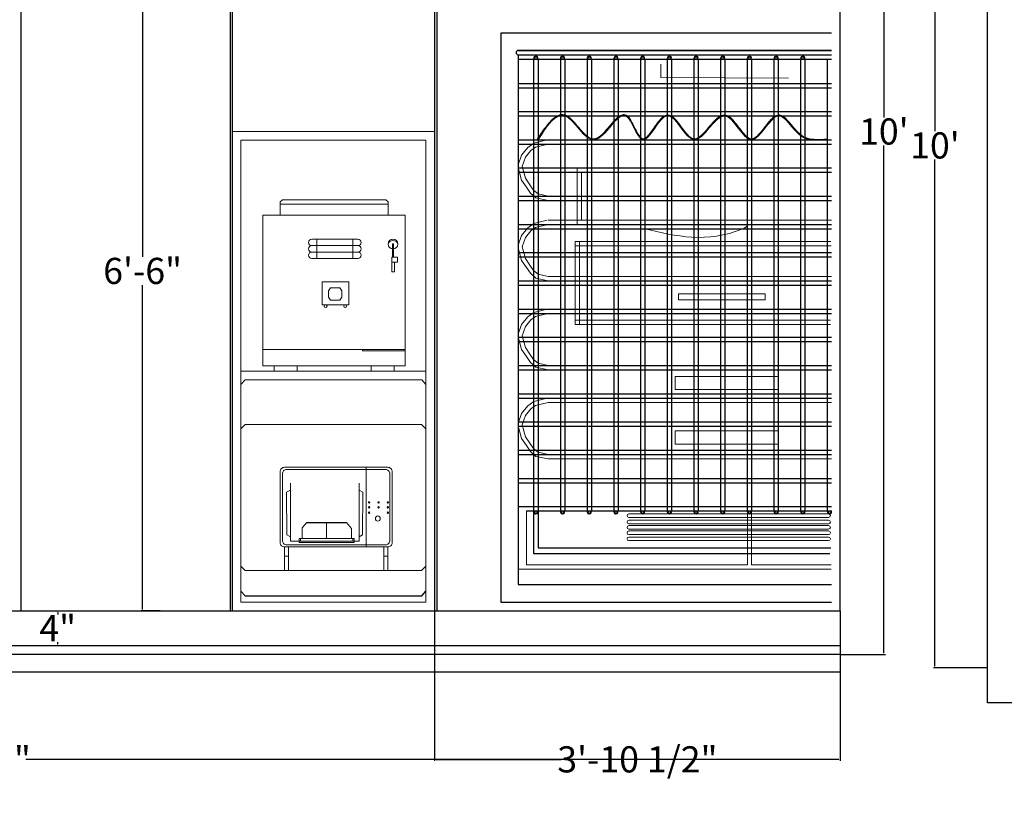
# Model space of a CAD drawing. Units: inches. Extents: x 1686244 to 1686928, y 1936095 to 1936489.
# Tile 5 of 11: x 1686365 to 1686478, y 1936336 to 1936425. Entities that reach past the tile are written whole.
import ezdxf

# ---------------------------------------------------------------- set-up
doc = ezdxf.new("R2010")
doc.units = ezdxf.units.IN
doc.header["$MEASUREMENT"] = 0
for name, color, linetype, lineweight in [('A-ANNO-DIMS', 240, 'Continuous', 18), ('A-ELEV', 7, 'Continuous', 25), ('A-ELEV-PATT', 72, 'Continuous', 13), ('A-FURN', 40, 'Continuous', 18)]:
    doc.layers.add(name, color=color, linetype=linetype, lineweight=lineweight)
doc.styles.get("Standard").update_dxf_attribs({"font": 'arial.ttf'})
doc.dimstyles.get("Standard").update_dxf_attribs({"dimtxt": 3, "dimasz": 0.18, "dimexe": 0.18, "dimexo": 0.0625, "dimgap": 0.09, "dimtad": 0, "dimtih": 1, "dimtoh": 1, "dimzin": 0, "dimdsep": 46, "dimlunit": 4, "dimtxsty": 'Standard', "dimcen": 0.09, "dimadec": 0, "dimazin": 0, "dimtfac": 1, "dimtofl": 0, "dimtmove": 0, "dimatfit": 3, "dimfxl": 1, "dimtolj": 1, "dimtzin": 0, "dimarcsym": 0})

# ---------------------------------------------------------------- blocks, each defined once
blk = doc.blocks.new('*D8')
at = {"layer": 'A-ANNO-DIMS', "color": 0, "lineweight": -2, "transparency": 16777216}
for p, q in [((1686381.35, 1936435.41), (1686379.15, 1936435.41)), ((1686379.33, 1936435.23), (1686379.33, 1936398.03)), ((1686379.33, 1936357.59), (1686379.33, 1936394.79)), ((1686381.35, 1936357.41), (1686379.15, 1936357.41))]:
    blk.add_line(p, q, dxfattribs=at)
at = {"layer": 'A-ANNO-DIMS', "color": 0, "transparency": 16777216}
for points in [[(1686379.3, 1936435.23), (1686379.36, 1936435.23), (1686379.33, 1936435.41)], [(1686379.3, 1936357.59), (1686379.36, 1936357.59), (1686379.33, 1936357.41)]]:
    blk.add_solid(points, dxfattribs=at)
at = {"layer": 'Defpoints', "color": 0, "transparency": 16777216}
for p in [(1686379.33, 1936435.41), (1686381.41, 1936435.41), (1686381.41, 1936357.41)]:
    blk.add_point(p, dxfattribs=at)
at = {"layer": 'A-ANNO-DIMS', "color": 0, "transparency": 16777216, "insert": (1686379.33, 1936396.41), "char_height": 3, "attachment_point": 5}
blk.add_mtext('\\A1;6\'-6"', dxfattribs=at)
blk = doc.blocks.new('*D20')
at = {"layer": 'A-ANNO-DIMS', "color": 0, "lineweight": -2, "transparency": 16777216}
for p, q in [((1686476.2, 1936470.86), (1686470.03, 1936470.86)), ((1686470.21, 1936470.68), (1686470.21, 1936412.44)), ((1686470.21, 1936351.04), (1686470.21, 1936409.19)), ((1686476.2, 1936350.86), (1686470.03, 1936350.86))]:
    blk.add_line(p, q, dxfattribs=at)
at = {"layer": 'A-ANNO-DIMS', "color": 0, "transparency": 16777216}
for points in [[(1686470.18, 1936470.68), (1686470.24, 1936470.68), (1686470.21, 1936470.86)], [(1686470.18, 1936351.04), (1686470.24, 1936351.04), (1686470.21, 1936350.86)]]:
    blk.add_solid(points, dxfattribs=at)
at = {"layer": 'Defpoints', "color": 0, "transparency": 16777216}
for p in [(1686476.26, 1936470.86), (1686470.21, 1936350.86), (1686476.26, 1936350.86)]:
    blk.add_point(p, dxfattribs=at)
at = {"layer": 'A-ANNO-DIMS', "color": 0, "transparency": 16777216, "insert": (1686470.21, 1936410.81), "char_height": 3, "attachment_point": 5}
blk.add_mtext("\\A1;10'", dxfattribs=at)
blk = doc.blocks.new('*D57')
at = {"layer": 'A-ANNO-DIMS', "color": 0, "lineweight": -2, "transparency": 16777216}
for p, q in [((1686368.79, 1936357.41), (1686369.77, 1936357.41)), ((1686369.59, 1936357.23), (1686369.59, 1936357)), ((1686368.79, 1936353.41), (1686369.77, 1936353.41)), ((1686369.59, 1936353.59), (1686369.59, 1936353.82))]:
    blk.add_line(p, q, dxfattribs=at)
at = {"layer": 'A-ANNO-DIMS', "color": 0, "transparency": 16777216}
for points in [[(1686369.56, 1936357.23), (1686369.62, 1936357.23), (1686369.59, 1936357.41)], [(1686369.56, 1936353.59), (1686369.62, 1936353.59), (1686369.59, 1936353.41)]]:
    blk.add_solid(points, dxfattribs=at)
at = {"layer": 'Defpoints', "color": 0, "transparency": 16777216}
for p in [(1686368.73, 1936357.41), (1686369.59, 1936357.41), (1686368.73, 1936353.41)]:
    blk.add_point(p, dxfattribs=at)
at = {"layer": 'A-ANNO-DIMS', "color": 0, "transparency": 16777216, "insert": (1686369.59, 1936355.41), "char_height": 3, "attachment_point": 5}
blk.add_mtext('\\A1;4"', dxfattribs=at)
blk = doc.blocks.new('*D64')
at = {"layer": 'A-ANNO-DIMS', "color": 0, "lineweight": -2, "transparency": 16777216}
for p, q in [((1686459.35, 1936472.41), (1686464.53, 1936472.41)), ((1686464.35, 1936472.23), (1686464.35, 1936414.03)), ((1686464.35, 1936352.59), (1686464.35, 1936410.79)), ((1686459.35, 1936352.41), (1686464.53, 1936352.41))]:
    blk.add_line(p, q, dxfattribs=at)
at = {"layer": 'A-ANNO-DIMS', "color": 0, "transparency": 16777216}
for points in [[(1686464.32, 1936472.23), (1686464.38, 1936472.23), (1686464.35, 1936472.41)], [(1686464.32, 1936352.59), (1686464.38, 1936352.59), (1686464.35, 1936352.41)]]:
    blk.add_solid(points, dxfattribs=at)
at = {"layer": 'Defpoints', "color": 0, "transparency": 16777216}
for p in [(1686459.29, 1936472.41), (1686459.29, 1936352.41), (1686464.35, 1936352.41)]:
    blk.add_point(p, dxfattribs=at)
at = {"layer": 'A-ANNO-DIMS', "color": 0, "transparency": 16777216, "insert": (1686464.35, 1936412.41), "char_height": 3, "attachment_point": 5}
blk.add_mtext("\\A1;10'", dxfattribs=at)
blk = doc.blocks.new('*D87')
at = {"layer": 'A-ANNO-DIMS', "color": 0, "lineweight": -2, "transparency": 16777216}
for p, q in [((1686262.35, 1936350.35), (1686262.35, 1936340.18)), ((1686459.35, 1936350.35), (1686459.35, 1936340.18)), ((1686262.53, 1936340.36), (1686355.75, 1936340.36)), ((1686459.17, 1936340.36), (1686365.95, 1936340.36))]:
    blk.add_line(p, q, dxfattribs=at)
at = {"layer": 'A-ANNO-DIMS', "color": 0, "transparency": 16777216}
for points in [[(1686262.53, 1936340.39), (1686262.53, 1936340.33), (1686262.35, 1936340.36)], [(1686459.17, 1936340.39), (1686459.17, 1936340.33), (1686459.35, 1936340.36)]]:
    blk.add_solid(points, dxfattribs=at)
at = {"layer": 'Defpoints', "color": 0, "transparency": 16777216}
for p in [(1686262.35, 1936350.41), (1686459.35, 1936350.41), (1686459.35, 1936340.36)]:
    blk.add_point(p, dxfattribs=at)
at = {"layer": 'A-ANNO-DIMS', "color": 0, "transparency": 16777216, "insert": (1686360.85, 1936340.36), "char_height": 3, "attachment_point": 5}
blk.add_mtext('\\A1;16\'-5"', dxfattribs=at)
blk = doc.blocks.new('*D91')
at = {"layer": 'A-ANNO-DIMS', "color": 0, "lineweight": -2, "transparency": 16777216}
for p, q in [((1686412.81, 1936357.35), (1686412.81, 1936340.18)), ((1686459.35, 1936357.35), (1686459.35, 1936340.18)), ((1686412.99, 1936340.36), (1686427.34, 1936340.36)), ((1686459.17, 1936340.36), (1686444.82, 1936340.36))]:
    blk.add_line(p, q, dxfattribs=at)
at = {"layer": 'A-ANNO-DIMS', "color": 0, "transparency": 16777216}
for points in [[(1686412.99, 1936340.39), (1686412.99, 1936340.33), (1686412.81, 1936340.36)], [(1686459.17, 1936340.39), (1686459.17, 1936340.33), (1686459.35, 1936340.36)]]:
    blk.add_solid(points, dxfattribs=at)
at = {"layer": 'Defpoints', "color": 0, "transparency": 16777216}
for p in [(1686412.81, 1936357.41), (1686459.35, 1936357.41), (1686459.35, 1936340.36)]:
    blk.add_point(p, dxfattribs=at)
at = {"layer": 'A-ANNO-DIMS', "color": 0, "transparency": 16777216, "insert": (1686436.08, 1936340.36), "char_height": 3, "attachment_point": 5}
blk.add_mtext('\\A1;3\'-10 1/2"', dxfattribs=at)

msp = doc.modelspace()

# ---------------------------------------------------------------- linework, layer by layer
at = {"layer": 'A-ELEV'}
for p, q in [((1686365.353, 1936467.412), (1686365.353, 1936357.412)), ((1686389.353, 1936467.412), (1686389.353, 1936357.412)), ((1686389.609, 1936467.412), (1686389.609, 1936357.412)), ((1686412.809, 1936467.412), (1686412.809, 1936357.412)), ((1686413.059, 1936467.412), (1686413.059, 1936357.412)), ((1686422.413, 1936421.704), (1686458.353, 1936421.704)), ((1686422.413, 1936421.204), (1686458.353, 1936421.204)), ((1686422.413, 1936420.704), (1686458.353, 1936420.704)), ((1686424.183, 1936420.704), (1686424.183, 1936368.86)), ((1686424.683, 1936420.704), (1686424.683, 1936368.86)), ((1686427.244, 1936420.704), (1686427.244, 1936368.86)), ((1686427.744, 1936420.704), (1686427.744, 1936368.86)), ((1686430.305, 1936420.704), (1686430.305, 1936368.86)), ((1686430.805, 1936420.704), (1686430.805, 1936368.86)), ((1686433.366, 1936420.704), (1686433.366, 1936368.86)), ((1686433.866, 1936420.704), (1686433.866, 1936368.86)), ((1686436.427, 1936420.704), (1686436.427, 1936368.86)), ((1686436.927, 1936420.704), (1686436.927, 1936368.86)), ((1686439.488, 1936420.704), (1686439.488, 1936368.86)), ((1686439.988, 1936420.704), (1686439.988, 1936368.86)), ((1686442.549, 1936420.704), (1686442.549, 1936368.86)), ((1686443.049, 1936420.704), (1686443.049, 1936368.86)), ((1686445.609, 1936420.704), (1686445.609, 1936368.86)), ((1686446.109, 1936420.704), (1686446.109, 1936368.86)), ((1686448.67, 1936420.704), (1686448.67, 1936368.86)), ((1686449.17, 1936420.704), (1686449.17, 1936368.86)), ((1686451.731, 1936420.704), (1686451.731, 1936368.86)), ((1686452.231, 1936420.704), (1686452.231, 1936368.86)), ((1686454.792, 1936420.704), (1686454.792, 1936368.86)), ((1686455.292, 1936420.704), (1686455.292, 1936368.86)), ((1686457.853, 1936420.704), (1686457.853, 1936368.86)), ((1686422.413, 1936417.909), (1686458.353, 1936417.909)), ((1686422.413, 1936417.409), (1686458.353, 1936417.409)), ((1686422.413, 1936414.704), (1686458.353, 1936414.704)), ((1686422.413, 1936414.204), (1686458.353, 1936414.204)), ((1686422.413, 1936411.465), (1686458.353, 1936411.465)), ((1686422.413, 1936410.965), (1686458.353, 1936410.965)), ((1686422.413, 1936408.226), (1686458.353, 1936408.226)), ((1686422.413, 1936407.726), (1686458.353, 1936407.726)), ((1686422.413, 1936404.987), (1686458.353, 1936404.987)), ((1686422.413, 1936404.487), (1686458.353, 1936404.487)), ((1686422.413, 1936401.748), (1686458.353, 1936401.748)), ((1686422.413, 1936401.248), (1686458.353, 1936401.248)), ((1686422.413, 1936398.51), (1686458.353, 1936398.51)), ((1686422.413, 1936398.01), (1686458.353, 1936398.01)), ((1686422.413, 1936395.271), (1686458.353, 1936395.271)), ((1686422.413, 1936394.771), (1686458.353, 1936394.771)), ((1686422.413, 1936392.032), (1686458.353, 1936392.032)), ((1686422.413, 1936391.532), (1686458.353, 1936391.532)), ((1686422.413, 1936388.793), (1686458.353, 1936388.793)), ((1686422.413, 1936388.293), (1686458.353, 1936388.293)), ((1686422.413, 1936385.554), (1686458.353, 1936385.554)), ((1686422.413, 1936385.054), (1686458.353, 1936385.054)), ((1686391.075, 1936383.912), (1686390.609, 1936383.372)), ((1686422.413, 1936382.315), (1686458.353, 1936382.315)), ((1686422.413, 1936381.815), (1686458.353, 1936381.815)), ((1686422.413, 1936379.076), (1686458.353, 1936379.076)), ((1686422.413, 1936378.576), (1686458.353, 1936378.576)), ((1686422.413, 1936375.838), (1686458.353, 1936375.838)), ((1686422.413, 1936375.338), (1686458.353, 1936375.338)), ((1686422.413, 1936372.599), (1686458.353, 1936372.599)), ((1686422.413, 1936372.099), (1686458.353, 1936372.099)), ((1686422.413, 1936369.36), (1686458.353, 1936369.36)), ((1686423.367, 1936368.86), (1686458.353, 1936368.86)), ((1686424.183, 1936368.86), (1686424.183, 1936364.397)), ((1686424.683, 1936369.36), (1686424.683, 1936364.626)), ((1686424.183, 1936364.397), (1686424.183, 1936363.992)), ((1686424.683, 1936364.626), (1686458.265, 1936364.626)), ((1686424.183, 1936363.992), (1686458.172, 1936363.992)), ((1686422.413, 1936360.412), (1686458.353, 1936360.412)), ((1686391.075, 1936359.109), (1686390.609, 1936359.648)), ((1686391.075, 1936359.109), (1686411.343, 1936359.109)), ((1686411.343, 1936359.109), (1686411.809, 1936359.648)), ((1686420.413, 1936358.412), (1686458.353, 1936358.412)), ((1686459.353, 1936357.412), (1686459.353, 1936350.412)), ((1686262.353, 1936353.412), (1686459.353, 1936353.412)), ((1686262.353, 1936352.412), (1686459.353, 1936352.412)), ((1686262.353, 1936350.412), (1686459.353, 1936350.412))]:
    msp.add_line(p, q, dxfattribs=at)
for points in [[(1686691.259, 1936346.864), (1686476.258, 1936346.864), (1686476.258, 1936474.864), (1686691.259, 1936474.864)], [(1686459.353, 1936357.412), (1686459.353, 1936467.412), (1686262.353, 1936467.412), (1686262.353, 1936357.412)]]:
    msp.add_lwpolyline(points, close=True, dxfattribs=at)
for points in [[(1686458.353, 1936423.704), (1686420.413, 1936423.704), (1686420.413, 1936358.412)], [(1686458.353, 1936421.704), (1686422.413, 1936421.704)], [(1686422.413, 1936421.204), (1686422.413, 1936360.412)]]:
    msp.add_lwpolyline(points, dxfattribs=at)
for centre in [(1686424.438, 1936420.891), (1686427.5, 1936420.891), (1686430.563, 1936420.891), (1686433.626, 1936420.891), (1686436.688, 1936420.891), (1686439.751, 1936420.891), (1686442.814, 1936420.891), (1686445.877, 1936420.891), (1686448.939, 1936420.891), (1686452.002, 1936420.891), (1686455.065, 1936420.891), (1686424.438, 1936368.673), (1686427.5, 1936368.673), (1686430.563, 1936368.673), (1686433.626, 1936368.673), (1686436.688, 1936368.673), (1686439.751, 1936368.673), (1686442.814, 1936368.673), (1686445.877, 1936368.673), (1686448.939, 1936368.673), (1686452.002, 1936368.673), (1686455.065, 1936368.673), (1686458.128, 1936368.673)]:
    msp.add_circle(centre, 0.187, dxfattribs=at)
for centre, start, end in [((1686422.413, 1936421.454), 90, 270), ((1686424.433, 1936420.704), 0, 180), ((1686427.494, 1936420.704), 0, 180), ((1686430.555, 1936420.704), 0, 180), ((1686433.616, 1936420.704), 0, 180), ((1686436.677, 1936420.704), 0, 180), ((1686439.738, 1936420.704), 0, 180), ((1686442.799, 1936420.704), 0, 180), ((1686445.859, 1936420.704), 0, 180), ((1686448.92, 1936420.704), 0, 180), ((1686451.981, 1936420.704), 0, 180), ((1686455.042, 1936420.704), 0, 180), ((1686424.433, 1936368.86), 180, 0), ((1686427.494, 1936368.86), 180, 0), ((1686430.555, 1936368.86), 180, 0), ((1686433.616, 1936368.86), 180, 0), ((1686436.677, 1936368.86), 180, 0), ((1686439.738, 1936368.86), 180, 0), ((1686442.799, 1936368.86), 180, 0), ((1686445.859, 1936368.86), 180, 0), ((1686448.92, 1936368.86), 180, 0), ((1686451.981, 1936368.86), 180, 0), ((1686455.042, 1936368.86), 180, 0), ((1686458.103, 1936368.86), 180, 0)]:
    msp.add_arc(centre, 0.25, start, end, dxfattribs=at)
at = {"layer": 'A-ELEV-PATT'}
for p, q in [((1686438.763, 1936420.144), (1686438.763, 1936418.618)), ((1686453.413, 1936418.543), (1686438.763, 1936418.618)), ((1686458.353, 1936411.465), (1686425.837, 1936411.465)), ((1686458.353, 1936410.965), (1686425.837, 1936410.965)), ((1686436.949, 1936411.62), (1686436.949, 1936399.785)), ((1686448.67, 1936410.965), (1686448.67, 1936402.248)), ((1686457.853, 1936408.226), (1686429.184, 1936408.226)), ((1686429.184, 1936408.226), (1686429.184, 1936401.748)), ((1686457.853, 1936407.726), (1686429.684, 1936407.726)), ((1686429.684, 1936407.726), (1686429.684, 1936402.248)), ((1686458.353, 1936404.987), (1686425.837, 1936404.987)), ((1686458.353, 1936404.487), (1686425.837, 1936404.487)), ((1686458.353, 1936402.248), (1686425.837, 1936402.248)), ((1686458.353, 1936401.748), (1686425.837, 1936401.748)), ((1686429.184, 1936401.748), (1686458.353, 1936401.748)), ((1686429.684, 1936402.248), (1686458.353, 1936402.248)), ((1686458.282, 1936399.785), (1686428.93, 1936399.785)), ((1686428.93, 1936399.785), (1686428.93, 1936390.251)), ((1686458.291, 1936399.285), (1686428.93, 1936399.285)), ((1686429.43, 1936399.785), (1686429.43, 1936390.251)), ((1686458.353, 1936395.771), (1686425.837, 1936395.771)), ((1686458.353, 1936395.271), (1686425.837, 1936395.271)), ((1686458.353, 1936392.032), (1686425.837, 1936392.032)), ((1686458.353, 1936391.532), (1686425.837, 1936391.532)), ((1686428.93, 1936390.751), (1686458.227, 1936390.751)), ((1686428.93, 1936390.251), (1686458.227, 1936390.251)), ((1686458.353, 1936385.554), (1686425.337, 1936385.554)), ((1686458.353, 1936385.054), (1686425.837, 1936385.054)), ((1686458.353, 1936381.815), (1686425.837, 1936381.815)), ((1686458.353, 1936381.315), (1686425.837, 1936381.315)), ((1686458.353, 1936375.338), (1686425.837, 1936375.338)), ((1686458.353, 1936374.838), (1686425.837, 1936374.838)), ((1686423.367, 1936362.687), (1686423.367, 1936368.86)), ((1686449.17, 1936368.86), (1686449.17, 1936362.687)), ((1686435.105, 1936368.531), (1686458.007, 1936368.531)), ((1686435.105, 1936368.118), (1686458.007, 1936368.118)), ((1686435.105, 1936367.797), (1686458.007, 1936367.797)), ((1686448.699, 1936362.687), (1686448.699, 1936368.531)), ((1686435.105, 1936367.385), (1686458.007, 1936367.385)), ((1686435.105, 1936367.19), (1686458.007, 1936367.19)), ((1686435.105, 1936366.777), (1686458.007, 1936366.777)), ((1686435.105, 1936366.567), (1686458.007, 1936366.567)), ((1686435.105, 1936366.155), (1686458.007, 1936366.155)), ((1686435.105, 1936365.868), (1686458.007, 1936365.868)), ((1686435.105, 1936365.455), (1686458.007, 1936365.455)), ((1686422.413, 1936362.187), (1686458.325, 1936362.187)), ((1686423.367, 1936362.687), (1686448.699, 1936362.687)), ((1686449.17, 1936362.687), (1686458.325, 1936362.687))]:
    msp.add_line(p, q, dxfattribs=at)
for points in [[(1686425.714, 1936411.45), (1686424.198, 1936411.064), (1686423.514, 1936410.585), (1686422.794, 1936409.697), (1686422.407, 1936408.569)], [(1686425.837, 1936410.965), (1686424.41, 1936410.602), (1686423.858, 1936410.216), (1686423.238, 1936409.451), (1686422.88, 1936408.407)], [(1686425.837, 1936404.487), (1686424.45, 1936404.782), (1686423.807, 1936405.349), (1686423.345, 1936406.016), (1686422.787, 1936406.821), (1686422.397, 1936408.277)], [(1686425.837, 1936404.987), (1686424.683, 1936405.242), (1686424.183, 1936405.683), (1686423.756, 1936406.301), (1686423.248, 1936407.035), (1686422.88, 1936408.407)], [(1686425.714, 1936402.233), (1686424.198, 1936401.848), (1686423.514, 1936401.369), (1686422.794, 1936400.481), (1686422.407, 1936399.352)], [(1686425.837, 1936401.748), (1686424.41, 1936401.386), (1686423.858, 1936400.999), (1686423.238, 1936400.235), (1686422.88, 1936399.19)], [(1686425.837, 1936395.271), (1686424.45, 1936395.565), (1686423.807, 1936396.132), (1686423.345, 1936396.8), (1686422.787, 1936397.605), (1686422.397, 1936399.061)], [(1686425.837, 1936395.771), (1686424.683, 1936396.026), (1686424.183, 1936396.467), (1686423.756, 1936397.084), (1686423.248, 1936397.818), (1686422.88, 1936399.19)], [(1686425.714, 1936392.016), (1686424.198, 1936391.631), (1686423.514, 1936391.152), (1686422.794, 1936390.264), (1686422.407, 1936389.136)], [(1686425.837, 1936391.532), (1686424.41, 1936391.169), (1686423.858, 1936390.783), (1686423.238, 1936390.018), (1686422.88, 1936388.974)], [(1686425.837, 1936385.054), (1686424.45, 1936385.349), (1686423.807, 1936385.916), (1686423.345, 1936386.583), (1686422.787, 1936387.388), (1686422.397, 1936388.844)], [(1686425.837, 1936385.554), (1686424.683, 1936385.809), (1686424.183, 1936386.25), (1686423.756, 1936386.868), (1686423.248, 1936387.602), (1686422.88, 1936388.974)], [(1686425.714, 1936381.8), (1686424.198, 1936381.415), (1686423.514, 1936380.936), (1686422.794, 1936380.048), (1686422.407, 1936378.919)], [(1686425.837, 1936381.315), (1686424.41, 1936380.953), (1686423.858, 1936380.566), (1686423.238, 1936379.802), (1686422.88, 1936378.757)], [(1686425.837, 1936374.838), (1686424.45, 1936375.132), (1686423.807, 1936375.699), (1686423.345, 1936376.366), (1686422.787, 1936377.172), (1686422.397, 1936378.628)], [(1686425.837, 1936375.338), (1686424.683, 1936375.593), (1686424.183, 1936376.034), (1686423.756, 1936376.651), (1686423.248, 1936377.385), (1686422.88, 1936378.757)]]:
    msp.add_lwpolyline(points, dxfattribs=at)
for points in [[(1686440.784, 1936393.79), (1686450.756, 1936393.79), (1686450.756, 1936393.104), (1686440.784, 1936393.104)], [(1686440.405, 1936384.298), (1686452.231, 1936384.298), (1686452.231, 1936382.8), (1686440.405, 1936382.8)], [(1686440.405, 1936378.041), (1686452.231, 1936378.041), (1686452.231, 1936376.543), (1686440.405, 1936376.543)]]:
    msp.add_lwpolyline(points, close=True, dxfattribs=at)
for centre, start, end in [((1686435.105, 1936368.324), 90, 270), ((1686435.105, 1936367.591), 90, 270), ((1686458.007, 1936368.324), 270, 90), ((1686458.007, 1936367.591), 270, 90), ((1686435.105, 1936366.983), 90, 270), ((1686435.105, 1936366.361), 90, 270), ((1686458.007, 1936366.983), 270, 90), ((1686458.007, 1936366.361), 270, 90), ((1686435.105, 1936365.662), 90, 270), ((1686458.007, 1936365.662), 270, 90)]:
    msp.add_arc(centre, 0.206, start, end, dxfattribs=at)
for points, knots in [([(1686424.6, 1936411.52), (1686424.753, 1936411.753), (1686424.906, 1936411.986), (1686425.367, 1936412.667), (1686425.675, 1936413.097), (1686426.257, 1936413.758), (1686426.53, 1936414.009), (1686427.035, 1936414.295), (1686427.267, 1936414.364), (1686427.736, 1936414.339), (1686427.969, 1936414.235), (1686428.417, 1936413.909), (1686428.635, 1936413.69), (1686429.072, 1936413.206), (1686429.291, 1936412.941), (1686429.782, 1936412.375), (1686430.055, 1936412.08), (1686430.533, 1936411.711), (1686430.738, 1936411.602), (1686431.091, 1936411.541), (1686431.244, 1936411.559), (1686431.686, 1936411.748), (1686431.988, 1936412.013), (1686432.59, 1936412.656), (1686432.892, 1936413.033), (1686433.381, 1936413.597), (1686433.573, 1936413.805), (1686433.925, 1936414.116), (1686434.086, 1936414.229), (1686434.396, 1936414.349), (1686434.547, 1936414.365), (1686434.834, 1936414.276), (1686434.964, 1936414.176), (1686435.201, 1936413.909), (1686435.31, 1936413.742), (1686435.624, 1936413.2), (1686435.817, 1936412.777), (1686436.142, 1936412.162), (1686436.273, 1936411.94), (1686436.484, 1936411.689), (1686436.564, 1936411.621), (1686436.71, 1936411.552), (1686436.773, 1936411.55), (1686436.931, 1936411.601), (1686437.022, 1936411.659), (1686437.216, 1936411.83), (1686437.318, 1936411.943), (1686437.679, 1936412.388), (1686437.949, 1936412.804), (1686438.409, 1936413.444), (1686438.593, 1936413.684), (1686438.926, 1936414.026), (1686439.074, 1936414.148), (1686439.344, 1936414.281), (1686439.464, 1936414.312), (1686439.702, 1936414.305), (1686439.82, 1936414.27), (1686440.143, 1936414.105), (1686440.342, 1936413.92), (1686440.733, 1936413.476), (1686440.925, 1936413.216), (1686441.364, 1936412.619), (1686441.611, 1936412.28), (1686442.049, 1936411.819), (1686442.24, 1936411.667), (1686442.578, 1936411.541), (1686442.73, 1936411.548), (1686443.068, 1936411.683), (1686443.248, 1936411.812), (1686443.778, 1936412.296), (1686444.138, 1936412.748), (1686444.781, 1936413.499), (1686445.064, 1936413.811), (1686445.524, 1936414.153), (1686445.698, 1936414.246), (1686446.011, 1936414.314), (1686446.148, 1936414.311), (1686446.41, 1936414.237), (1686446.535, 1936414.169), (1686447.02, 1936413.815), (1686447.357, 1936413.368), (1686448.026, 1936412.477), (1686448.358, 1936412.033), (1686448.808, 1936411.676), (1686448.938, 1936411.605), (1686449.184, 1936411.551), (1686449.304, 1936411.568), (1686449.562, 1936411.684), (1686449.7, 1936411.784), (1686449.981, 1936412.044), (1686450.124, 1936412.204), (1686450.594, 1936412.775), (1686450.924, 1936413.246), (1686451.439, 1936413.833), (1686451.621, 1936414.014), (1686451.954, 1936414.233), (1686452.104, 1936414.294), (1686452.409, 1936414.317), (1686452.559, 1936414.275), (1686452.843, 1936414.124), (1686452.979, 1936414.016), (1686453.374, 1936413.64), (1686453.629, 1936413.316), (1686454.164, 1936412.669), (1686454.441, 1936412.347), (1686454.975, 1936411.91), (1686455.229, 1936411.77), (1686455.763, 1936411.583), (1686456.043, 1936411.533), (1686456.817, 1936411.477), (1686457.328, 1936411.52), (1686457.844, 1936411.565)], [0, 0, 0, 0, 0.6198497, 0.6198497, 1.8595491, 1.8595491, 2.9317453, 2.9317453, 3.7773121, 3.7773121, 4.6228788, 4.6228788, 5.4684455, 5.4684455, 6.3140123, 6.3140123, 7.3654424, 7.3654424, 8.1736983, 8.1736983, 8.812576, 8.812576, 9.9067512, 9.9067512, 11.0009263, 11.0009263, 11.7236696, 11.7236696, 12.3447229, 12.3447229, 12.8877348, 12.8877348, 13.4307466, 13.4307466, 13.9737585, 13.9737585, 15.0258606, 15.0258606, 15.7385229, 15.7385229, 16.195193, 16.195193, 16.6560278, 16.6560278, 17.1168626, 17.1168626, 17.5776974, 17.5776974, 18.6933699, 18.6933699, 19.4222939, 19.4222939, 19.9794482, 19.9794482, 20.3901997, 20.3901997, 20.8009512, 20.8009512, 21.5807194, 21.5807194, 22.3604876, 22.3604876, 23.3657967, 23.3657967, 24.1584136, 24.1584136, 24.8711455, 24.8711455, 25.5838774, 25.5838774, 26.9255116, 26.9255116, 27.9769724, 27.9769724, 28.5946697, 28.5946697, 29.0495877, 29.0495877, 29.5045058, 29.5045058, 30.8620561, 30.8620561, 32.2196063, 32.2196063, 32.798175, 32.798175, 33.3767438, 33.3767438, 33.9553125, 33.9553125, 34.5338812, 34.5338812, 35.8487479, 35.8487479, 36.5727796, 36.5727796, 37.1250725, 37.1250725, 37.6773653, 37.6773653, 38.2296582, 38.2296582, 39.294376, 39.294376, 40.3590938, 40.3590938, 41.2411052, 41.2411052, 42.1231167, 42.1231167, 43.5982821, 43.5982821, 43.5982821, 43.5982821]), ([(1686424.621, 1936411.506), (1686424.774, 1936411.739), (1686424.927, 1936411.972), (1686425.387, 1936412.652), (1686425.695, 1936413.081), (1686426.29, 1936413.758), (1686426.578, 1936414.018), (1686427.097, 1936414.291), (1686427.328, 1936414.348), (1686427.792, 1936414.295), (1686428.021, 1936414.177), (1686428.468, 1936413.828), (1686428.688, 1936413.598), (1686429.321, 1936412.884), (1686429.736, 1936412.351), (1686430.369, 1936411.791), (1686430.588, 1936411.645), (1686430.977, 1936411.519), (1686431.148, 1936411.515), (1686431.612, 1936411.664), (1686431.919, 1936411.915), (1686432.531, 1936412.547), (1686432.838, 1936412.928), (1686433.342, 1936413.515), (1686433.542, 1936413.738), (1686433.911, 1936414.074), (1686434.081, 1936414.198), (1686434.379, 1936414.317), (1686434.508, 1936414.336), (1686434.76, 1936414.283), (1686434.878, 1936414.21), (1686435.095, 1936414.002), (1686435.196, 1936413.866), (1686435.53, 1936413.342), (1686435.746, 1936412.863), (1686436.093, 1936412.198), (1686436.224, 1936411.971), (1686436.443, 1936411.693), (1686436.533, 1936411.611), (1686436.699, 1936411.527), (1686436.776, 1936411.523), (1686436.954, 1936411.584), (1686437.054, 1936411.651), (1686437.266, 1936411.846), (1686437.377, 1936411.972), (1686437.767, 1936412.469), (1686438.059, 1936412.926), (1686438.53, 1936413.559), (1686438.703, 1936413.772), (1686439.057, 1936414.106), (1686439.239, 1936414.228), (1686439.58, 1936414.302), (1686439.733, 1936414.277), (1686440.021, 1936414.146), (1686440.16, 1936414.042), (1686440.557, 1936413.667), (1686440.81, 1936413.329), (1686441.318, 1936412.64), (1686441.571, 1936412.289), (1686442.008, 1936411.823), (1686442.191, 1936411.671), (1686442.542, 1936411.518), (1686442.71, 1936411.517), (1686443.073, 1936411.654), (1686443.264, 1936411.791), (1686443.654, 1936412.15), (1686443.853, 1936412.371), (1686444.411, 1936413.022), (1686444.772, 1936413.479), (1686445.34, 1936413.999), (1686445.545, 1936414.147), (1686445.897, 1936414.275), (1686446.04, 1936414.294), (1686446.429, 1936414.229), (1686446.659, 1936414.07), (1686447.106, 1936413.641), (1686447.323, 1936413.368), (1686447.791, 1936412.751), (1686448.042, 1936412.403), (1686448.476, 1936411.912), (1686448.66, 1936411.74), (1686448.977, 1936411.562), (1686449.108, 1936411.528), (1686449.374, 1936411.56), (1686449.512, 1936411.625), (1686449.801, 1936411.834), (1686449.95, 1936411.978), (1686450.568, 1936412.664), (1686451.041, 1936413.402), (1686451.676, 1936414.019), (1686451.836, 1936414.143), (1686452.127, 1936414.269), (1686452.256, 1936414.293), (1686452.508, 1936414.264), (1686452.63, 1936414.216), (1686453.054, 1936413.958), (1686453.343, 1936413.623), (1686453.947, 1936412.894), (1686454.259, 1936412.499), (1686454.782, 1936412.024), (1686454.978, 1936411.886), (1686455.387, 1936411.679), (1686455.599, 1936411.608), (1686456.258, 1936411.463), (1686456.726, 1936411.462), (1686457.417, 1936411.503), (1686457.631, 1936411.521), (1686457.846, 1936411.54)], [0, 0, 0, 0, 0.6195688, 0.6195688, 1.8587065, 1.8587065, 2.9947443, 2.9947443, 3.8509643, 3.8509643, 4.7071842, 4.7071842, 5.5634041, 5.5634041, 7.1611739, 7.1611739, 8.0023315, 8.0023315, 8.6973238, 8.6973238, 9.8074601, 9.8074601, 10.9175963, 10.9175963, 11.6720865, 11.6720865, 12.3339957, 12.3339957, 12.8235788, 12.8235788, 13.3131619, 13.3131619, 13.802745, 13.802745, 14.9803996, 14.9803996, 15.6853017, 15.6853017, 16.1753468, 16.1753468, 16.6653918, 16.6653918, 17.1554369, 17.1554369, 17.645482, 17.645482, 18.8425445, 18.8425445, 19.5256228, 19.5256228, 20.208701, 20.208701, 20.7473398, 20.7473398, 21.2859785, 21.2859785, 22.3167922, 22.3167922, 23.3476058, 23.3476058, 24.0974736, 24.0974736, 24.8473414, 24.8473414, 25.5972092, 25.5972092, 26.347077, 26.347077, 27.6906732, 27.6906732, 28.4455681, 28.4455681, 28.9435164, 28.9435164, 29.8123427, 29.8123427, 30.6811689, 30.6811689, 31.706993, 31.706993, 32.4760399, 32.4760399, 33.0780575, 33.0780575, 33.6800751, 33.6800751, 34.2820927, 34.2820927, 36.1683264, 36.1683264, 36.8029374, 36.8029374, 37.2799861, 37.2799861, 37.7570348, 37.7570348, 38.9828061, 38.9828061, 40.2085774, 40.2085774, 40.9022496, 40.9022496, 41.5959217, 41.5959217, 42.9832661, 42.9832661, 43.5982821, 43.5982821, 43.5982821, 43.5982821]), ([(1686424.642, 1936411.492), (1686424.795, 1936411.725), (1686424.948, 1936411.958), (1686425.407, 1936412.637), (1686425.714, 1936413.065), (1686426.332, 1936413.767), (1686426.642, 1936414.042), (1686427.185, 1936414.292), (1686427.416, 1936414.331), (1686427.878, 1936414.233), (1686428.105, 1936414.093), (1686428.555, 1936413.707), (1686428.779, 1936413.462), (1686429.425, 1936412.716), (1686429.851, 1936412.18), (1686430.493, 1936411.677), (1686430.706, 1936411.56), (1686431.069, 1936411.492), (1686431.22, 1936411.505), (1686431.533, 1936411.622), (1686431.694, 1936411.723), (1686432.331, 1936412.237), (1686432.816, 1936412.874), (1686433.549, 1936413.71), (1686433.811, 1936413.981), (1686434.225, 1936414.242), (1686434.382, 1936414.301), (1686434.653, 1936414.293), (1686434.767, 1936414.249), (1686434.978, 1936414.092), (1686435.077, 1936413.981), (1686435.442, 1936413.474), (1686435.686, 1936412.926), (1686436.086, 1936412.156), (1686436.241, 1936411.888), (1686436.493, 1936411.611), (1686436.587, 1936411.542), (1686436.769, 1936411.496), (1686436.863, 1936411.515), (1686437.07, 1936411.629), (1686437.182, 1936411.726), (1686437.412, 1936411.973), (1686437.53, 1936412.123), (1686437.97, 1936412.721), (1686438.306, 1936413.252), (1686438.821, 1936413.859), (1686438.997, 1936414.031), (1686439.304, 1936414.215), (1686439.434, 1936414.259), (1686439.695, 1936414.259), (1686439.823, 1936414.217), (1686440.246, 1936413.979), (1686440.531, 1936413.647), (1686441.102, 1936412.901), (1686441.386, 1936412.486), (1686441.859, 1936411.933), (1686442.048, 1936411.75), (1686442.372, 1936411.552), (1686442.507, 1936411.507), (1686442.781, 1936411.512), (1686442.921, 1936411.559), (1686443.365, 1936411.812), (1686443.677, 1936412.133), (1686444.375, 1936412.935), (1686444.763, 1936413.436), (1686445.359, 1936413.983), (1686445.569, 1936414.133), (1686445.918, 1936414.254), (1686446.056, 1936414.269), (1686446.327, 1936414.218), (1686446.459, 1936414.155), (1686446.929, 1936413.833), (1686447.253, 1936413.421), (1686447.896, 1936412.569), (1686448.214, 1936412.128), (1686448.715, 1936411.67), (1686448.899, 1936411.555), (1686449.254, 1936411.492), (1686449.432, 1936411.549), (1686449.808, 1936411.798), (1686450.001, 1936411.99), (1686450.58, 1936412.66), (1686450.968, 1936413.233), (1686451.543, 1936413.868), (1686451.731, 1936414.042), (1686452.054, 1936414.22), (1686452.186, 1936414.261), (1686452.545, 1936414.253), (1686452.759, 1936414.13), (1686453.182, 1936413.768), (1686453.392, 1936413.525), (1686453.829, 1936412.997), (1686454.056, 1936412.712), (1686454.471, 1936412.268), (1686454.653, 1936412.096), (1686455.293, 1936411.636), (1686455.792, 1936411.503), (1686456.811, 1936411.425), (1686457.329, 1936411.47), (1686457.848, 1936411.515)], [0, 0, 0, 0, 0.6193174, 0.6193174, 1.8579521, 1.8579521, 3.0912244, 3.0912244, 3.9643916, 3.9643916, 4.8375588, 4.8375588, 5.710726, 5.710726, 7.3459362, 7.3459362, 8.1613339, 8.1613339, 8.7505031, 8.7505031, 9.3396724, 9.3396724, 11.0678935, 11.0678935, 12.0793947, 12.0793947, 12.6988845, 12.6988845, 13.1669126, 13.1669126, 13.6349408, 13.6349408, 14.9631998, 14.9631998, 15.7997297, 15.7997297, 16.3113985, 16.3113985, 16.8230673, 16.8230673, 17.3347361, 17.3347361, 17.8464048, 17.8464048, 19.1981438, 19.1981438, 19.886515, 19.886515, 20.3687926, 20.3687926, 20.8510702, 20.8510702, 22.0086987, 22.0086987, 23.1663272, 23.1663272, 23.9272524, 23.9272524, 24.4976466, 24.4976466, 25.0680408, 25.0680408, 26.2451429, 26.2451429, 27.6882844, 27.6882844, 28.4651476, 28.4651476, 28.9599931, 28.9599931, 29.4548387, 29.4548387, 30.7578931, 30.7578931, 32.0609476, 32.0609476, 32.8352107, 32.8352107, 33.6094739, 33.6094739, 34.383737, 34.383737, 35.9290421, 35.9290421, 36.685788, 36.685788, 37.2013603, 37.2013603, 38.0798613, 38.0798613, 38.9583623, 38.9583623, 39.8595949, 39.8595949, 40.5263588, 40.5263588, 42.1123246, 42.1123246, 43.5982821, 43.5982821, 43.5982821, 43.5982821]), ([(1686424.663, 1936411.479), (1686424.815, 1936411.711), (1686424.968, 1936411.944), (1686425.427, 1936412.623), (1686425.734, 1936413.05), (1686426.386, 1936413.791), (1686426.733, 1936414.087), (1686427.316, 1936414.295), (1686427.55, 1936414.303), (1686428.016, 1936414.13), (1686428.246, 1936413.954), (1686428.974, 1936413.253), (1686429.476, 1936412.558), (1686430.221, 1936411.842), (1686430.458, 1936411.66), (1686430.906, 1936411.474), (1686431.117, 1936411.454), (1686431.548, 1936411.589), (1686431.769, 1936411.739), (1686432.486, 1936412.375), (1686432.984, 1936413.049), (1686433.735, 1936413.865), (1686434.007, 1936414.114), (1686434.401, 1936414.272), (1686434.532, 1936414.288), (1686434.897, 1936414.186), (1686435.106, 1936413.929), (1686435.505, 1936413.267), (1686435.694, 1936412.861), (1686436.011, 1936412.244), (1686436.139, 1936412.013), (1686436.395, 1936411.663), (1686436.523, 1936411.542), (1686436.777, 1936411.459), (1686436.909, 1936411.497), (1686437.196, 1936411.697), (1686437.348, 1936411.858), (1686437.86, 1936412.499), (1686438.238, 1936413.121), (1686438.803, 1936413.804), (1686438.984, 1936413.987), (1686439.294, 1936414.184), (1686439.423, 1936414.231), (1686439.68, 1936414.237), (1686439.807, 1936414.197), (1686440.21, 1936413.972), (1686440.481, 1936413.666), (1686441.023, 1936412.967), (1686441.293, 1936412.573), (1686441.753, 1936412.011), (1686441.941, 1936411.812), (1686442.281, 1936411.566), (1686442.433, 1936411.498), (1686442.736, 1936411.475), (1686442.891, 1936411.519), (1686443.373, 1936411.778), (1686443.708, 1936412.128), (1686444.38, 1936412.906), (1686444.718, 1936413.334), (1686445.255, 1936413.863), (1686445.456, 1936414.027), (1686445.817, 1936414.206), (1686445.98, 1936414.245), (1686446.302, 1936414.206), (1686446.459, 1936414.131), (1686446.949, 1936413.774), (1686447.274, 1936413.353), (1686447.919, 1936412.495), (1686448.24, 1936412.057), (1686448.746, 1936411.618), (1686448.933, 1936411.511), (1686449.302, 1936411.474), (1686449.489, 1936411.547), (1686449.871, 1936411.822), (1686450.065, 1936412.022), (1686450.771, 1936412.855), (1686451.282, 1936413.658), (1686451.974, 1936414.168), (1686452.163, 1936414.245), (1686452.537, 1936414.217), (1686452.719, 1936414.121), (1686453.08, 1936413.83), (1686453.26, 1936413.636), (1686453.687, 1936413.135), (1686453.937, 1936412.814), (1686454.392, 1936412.31), (1686454.592, 1936412.113), (1686455.221, 1936411.649), (1686455.682, 1936411.507), (1686456.707, 1936411.391), (1686457.278, 1936411.44), (1686457.851, 1936411.49)], [0, 0, 0, 0, 0.6191078, 0.6191078, 1.8573235, 1.8573235, 3.2418915, 3.2418915, 4.1465272, 4.1465272, 5.051163, 5.051163, 6.9951759, 6.9951759, 7.8879589, 7.8879589, 8.6854056, 8.6854056, 9.4828522, 9.4828522, 11.2647437, 11.2647437, 12.3306937, 12.3306937, 12.8732152, 12.8732152, 13.8945556, 13.8945556, 14.915896, 14.915896, 15.6061768, 15.6061768, 16.2732019, 16.2732019, 16.9402269, 16.9402269, 17.607252, 17.607252, 19.1409727, 19.1409727, 19.856223, 19.856223, 20.3517613, 20.3517613, 20.8472996, 20.8472996, 21.9483472, 21.9483472, 23.0493947, 23.0493947, 23.8052513, 23.8052513, 24.417441, 24.417441, 25.0296308, 25.0296308, 26.2884347, 26.2884347, 27.5472385, 27.5472385, 28.2985943, 28.2985943, 28.9020839, 28.9020839, 29.5055734, 29.5055734, 30.8152318, 30.8152318, 32.1248902, 32.1248902, 32.8982906, 32.8982906, 33.6716909, 33.6716909, 34.4450913, 34.4450913, 36.4854523, 36.4854523, 37.2441814, 37.2441814, 38.0029104, 38.0029104, 38.7616394, 38.7616394, 39.762661, 39.762661, 40.4957963, 40.4957963, 41.962067, 41.962067, 43.5982821, 43.5982821, 43.5982821, 43.5982821]), ([(1686424.683, 1936411.465), (1686425.697, 1936413.008), (1686427.8, 1936416.207), (1686431.128, 1936408.7), (1686434.744, 1936416.895), (1686436.62, 1936408.943), (1686439.577, 1936416.96), (1686442.564, 1936408.597), (1686446.093, 1936417.016), (1686449.131, 1936408.827), (1686452.137, 1936416.274), (1686454.49, 1936411.174), (1686456.77, 1936411.371), (1686457.853, 1936411.465)], [0, 0, 0, 0, 4.1073188, 8.5171761, 12.977427, 16.3503, 20.2659148, 24.3732336, 28.8655509, 32.9728697, 37.0801885, 40.5015696, 43.5982821, 43.5982821, 43.5982821, 43.5982821]), ([(1686436.949, 1936401.248), (1686440.495, 1936400.388), (1686444.247, 1936399.478), (1686448.682, 1936401.471), (1686448.671, 1936401.72), (1686448.67, 1936401.748)], [0, 0, 0, 0, 11.2208875, 11.8717764, 11.9550553, 11.9550553, 11.9550553, 11.9550553])]:
    msp.add_open_spline(points, degree=3, knots=knots, dxfattribs=at)
at = {"layer": 'A-FURN'}
for p, q in [((1686395.09, 1936404.322), (1686395.367, 1936404.564)), ((1686395.09, 1936404.081), (1686395.09, 1936404.322)), ((1686395.367, 1936404.564), (1686407.221, 1936404.564)), ((1686407.498, 1936404.322), (1686407.221, 1936404.564)), ((1686407.498, 1936404.322), (1686407.498, 1936404.081)), ((1686398.725, 1936400.044), (1686404.019, 1936400.044)), ((1686398.725, 1936399.31), (1686404.019, 1936399.31)), ((1686407.998, 1936399.484), (1686407.998, 1936397.989)), ((1686408.098, 1936399.484), (1686408.098, 1936397.989)), ((1686398.725, 1936398.575), (1686404.019, 1936398.575)), ((1686398.725, 1936397.84), (1686404.019, 1936397.84)), ((1686407.902, 1936397.417), (1686407.902, 1936396.298)), ((1686408.213, 1936396.298), (1686408.213, 1936397.417)), ((1686407.902, 1936396.298), (1686408.213, 1936396.298)), ((1686400.639, 1936394.11), (1686400.862, 1936394.469)), ((1686402.177, 1936394.11), (1686401.954, 1936394.469)), ((1686400.639, 1936393.416), (1686400.862, 1936393.056)), ((1686402.177, 1936393.416), (1686401.954, 1936393.056)), ((1686393.127, 1936387.408), (1686409.46, 1936387.408)), ((1686390.609, 1936384.912), (1686411.809, 1936384.912)), ((1686394.409, 1936385.499), (1686394.409, 1936384.912)), ((1686394.409, 1936384.912), (1686397.059, 1936384.912)), ((1686397.059, 1936384.912), (1686397.059, 1936385.499)), ((1686405.528, 1936384.912), (1686405.528, 1936385.499)), ((1686408.178, 1936384.912), (1686405.528, 1936384.912)), ((1686408.178, 1936385.499), (1686408.178, 1936384.912)), ((1686391.075, 1936383.912), (1686411.343, 1936383.912)), ((1686411.343, 1936383.912), (1686411.809, 1936383.372)), ((1686404.952, 1936373.87), (1686404.952, 1936364.728)), ((1686404.977, 1936373.87), (1686404.977, 1936364.728)), ((1686396.275, 1936371.245), (1686395.842, 1936371.013)), ((1686395.842, 1936371.013), (1686395.873, 1936366.126)), ((1686396.275, 1936372.041), (1686396.275, 1936365.395)), ((1686404.154, 1936372.041), (1686404.154, 1936365.395)), ((1686404.154, 1936371.245), (1686404.587, 1936371.013)), ((1686404.587, 1936371.013), (1686404.556, 1936366.126)), ((1686397.624, 1936366.921), (1686398.164, 1936367.537)), ((1686397.624, 1936365.712), (1686397.624, 1936366.921)), ((1686398.136, 1936367.505), (1686402.743, 1936367.504)), ((1686398.164, 1936367.537), (1686402.714, 1936367.537)), ((1686400.439, 1936365.712), (1686400.439, 1936367.537)), ((1686403.304, 1936366.864), (1686402.714, 1936367.537)), ((1686403.304, 1936366.864), (1686403.304, 1936365.712)), ((1686396.275, 1936365.91), (1686395.873, 1936366.126)), ((1686396.275, 1936365.395), (1686404.154, 1936365.395)), ((1686397.288, 1936365.712), (1686397.288, 1936365.244)), ((1686403.589, 1936365.712), (1686397.288, 1936365.712)), ((1686397.442, 1936365.713), (1686397.442, 1936365.396)), ((1686403.436, 1936365.712), (1686403.436, 1936365.395)), ((1686403.589, 1936365.244), (1686403.589, 1936365.712)), ((1686404.154, 1936365.91), (1686404.556, 1936366.126)), ((1686397.288, 1936365.244), (1686403.589, 1936365.244)), ((1686395.607, 1936363.683), (1686395.607, 1936362.027)), ((1686396.07, 1936363.683), (1686396.07, 1936362.027)), ((1686406.981, 1936363.683), (1686406.981, 1936362.027)), ((1686407.445, 1936363.683), (1686407.445, 1936362.027))]:
    msp.add_line(p, q, dxfattribs=at)
for points in [[(1686389.609, 1936412.412), (1686412.809, 1936412.412), (1686412.809, 1936357.412), (1686389.609, 1936357.412), (1686389.609, 1936412.412)], [(1686400.639, 1936393.416), (1686400.639, 1936394.11)], [(1686400.862, 1936394.469), (1686401.954, 1936394.469)], [(1686402.177, 1936394.11), (1686402.177, 1936393.416)], [(1686401.954, 1936393.056), (1686400.862, 1936393.056)], [(1686409.46, 1936387.248), (1686404.54, 1936387.248), (1686404.54, 1936387.408)]]:
    msp.add_lwpolyline(points, dxfattribs=at)
for points in [[(1686390.609, 1936411.412), (1686411.809, 1936411.412), (1686411.809, 1936358.412), (1686390.609, 1936358.412)], [(1686395.09, 1936402.806), (1686407.498, 1936402.806), (1686407.498, 1936404.081), (1686395.09, 1936404.081)], [(1686393.127, 1936402.806), (1686409.46, 1936402.806), (1686409.46, 1936385.499), (1686393.127, 1936385.499)], [(1686399.32, 1936400.044), (1686403.424, 1936400.044), (1686403.424, 1936397.84), (1686399.32, 1936397.84)], [(1686407.902, 1936397.989), (1686408.554, 1936397.989), (1686408.554, 1936397.417), (1686407.902, 1936397.417)], [(1686399.92, 1936395.138), (1686402.97, 1936395.138), (1686402.97, 1936392.536), (1686399.92, 1936392.536)], [(1686391.109, 1936378.783), (1686411.309, 1936378.783), (1686411.809, 1936378.283), (1686411.809, 1936362.527), (1686411.309, 1936362.027), (1686391.109, 1936362.027), (1686390.609, 1936362.527), (1686390.609, 1936378.283)], [(1686395.607, 1936364.728), (1686396.07, 1936364.728), (1686396.07, 1936363.683), (1686395.607, 1936363.683)], [(1686407.445, 1936364.728), (1686406.981, 1936364.728), (1686406.981, 1936363.683), (1686407.445, 1936363.683)]]:
    msp.add_lwpolyline(points, close=True, dxfattribs=at)
for points in [[(1686395.607, 1936373.87), (1686407.445, 1936373.87, -0.4142136), (1686407.945, 1936373.37), (1686407.945, 1936365.228, -0.4142136), (1686407.445, 1936364.728), (1686395.607, 1936364.728, -0.4142136), (1686395.107, 1936365.228), (1686395.107, 1936373.37, -0.4142136)], [(1686395.857, 1936373.62), (1686407.195, 1936373.62, -0.4142136), (1686407.695, 1936373.12), (1686407.695, 1936365.478, -0.4142136), (1686407.195, 1936364.978), (1686395.857, 1936364.978, -0.4142136), (1686395.357, 1936365.478), (1686395.357, 1936373.12, -0.4142136)]]:
    msp.add_lwpolyline(points, format="xyb", close=True, dxfattribs=at)
for centre, radius in [((1686408.048, 1936399.484), 0.565), ((1686408.048, 1936399.484), 0.05), ((1686400.322, 1936392.367), 0.164), ((1686402.568, 1936392.367), 0.164), ((1686405.307, 1936369.835), 0.0808), ((1686406.388, 1936369.835), 0.0808), ((1686407.469, 1936369.835), 0.0808), ((1686405.307, 1936369.276), 0.0808), ((1686405.307, 1936368.667), 0.0808), ((1686406.388, 1936369.276), 0.0808), ((1686407.469, 1936369.276), 0.0808), ((1686407.469, 1936368.667), 0.0808)]:
    msp.add_circle(centre, radius, dxfattribs=at)
for centre, radius, start, end in [((1686398.725, 1936399.677), 0.367, 90, 270), ((1686398.725, 1936398.942), 0.367, 90, 270), ((1686404.019, 1936399.677), 0.367, 270, 90), ((1686404.019, 1936398.942), 0.367, 270, 90), ((1686408.048, 1936399.318), 0.589, 16.37294, 163.62706), ((1686398.725, 1936398.207), 0.367, 90, 270), ((1686404.019, 1936398.207), 0.367, 270, 90)]:
    msp.add_arc(centre, radius, start, end, dxfattribs=at)
msp.add_ellipse((1686406.312, 1936367.99), major_axis=(0, -0.299), ratio=0.9265496, start_param=-1.5707963, end_param=4.712389, dxfattribs=at)

# ---------------------------------------------------------------- dimensions: what is measured, and where the dimension line sits
at = {"layer": 'A-ANNO-DIMS'}
for base, p1, p2, picture, middle in [((1686464.354, 1936352.412), (1686459.29, 1936472.412), (1686459.29, 1936352.412), '*D64', (1686464.354, 1936412.412)), ((1686470.215, 1936350.864), (1686476.258, 1936470.864), (1686476.258, 1936350.864), '*D20', (1686470.215, 1936410.814))]:
    dim = msp.add_linear_dim(base=base, p1=p1, p2=p2, angle=90, dimstyle='Standard', override={"dimclrd": 0, "dimclre": 0, "dimclrt": 0}, dxfattribs=at)
    dim.commit()
    dim.dimension.update_dxf_attribs({"geometry": picture, "text_midpoint": middle, "dimtype": 160})
for base, p1, p2, picture, middle in [((1686379.328, 1936435.412), (1686381.411, 1936357.412), (1686381.411, 1936435.412), '*D8', (1686379.328, 1936396.412)), ((1686369.588, 1936357.412), (1686368.732, 1936353.412), (1686368.732, 1936357.412), '*D57', (1686369.588, 1936355.412))]:
    dim = msp.add_linear_dim(base=base, p1=p1, p2=p2, angle=90, dimstyle='Standard', override={"dimclrd": 0, "dimclre": 0, "dimclrt": 0}, dxfattribs=at)
    dim.commit()
    dim.dimension.update_dxf_attribs({"geometry": picture, "text_midpoint": middle})
for p1, p2, picture, middle in [((1686412.809, 1936357.412), (1686459.353, 1936357.412), '*D91', (1686436.081, 1936340.362)), ((1686262.353, 1936350.412), (1686459.353, 1936350.412), '*D87', (1686360.853, 1936340.362))]:
    dim = msp.add_linear_dim(base=(1686459.353, 1936340.362), p1=p1, p2=p2, dimstyle='Standard', override={"dimdec": 1, "dimlfac": 1, "dimrnd": 0, "dimzin": 1, "dimdsep": 46, "dimlunit": 4, "dimfrac": 2}, dxfattribs=at)
    dim.commit()
    dim.dimension.update_dxf_attribs({"geometry": picture, "text_midpoint": middle})

doc.saveas('drawing.dxf')
